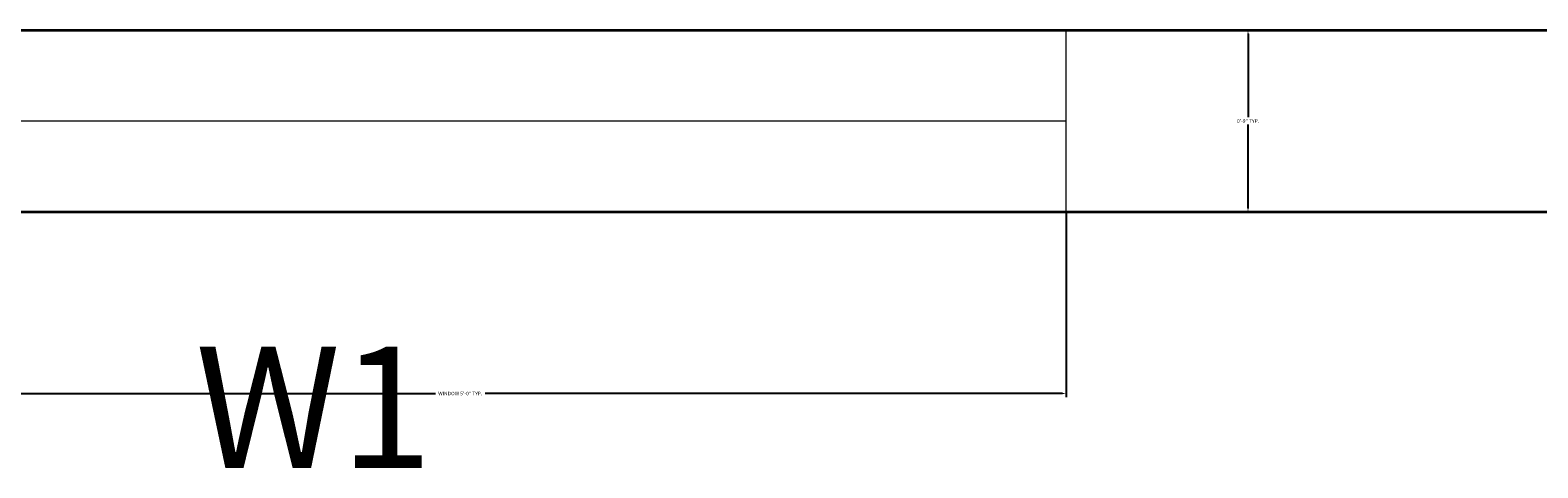
# Model space of a CAD drawing. Units: inches. Extents: x -36302355 to 648, y -221479757 to 75.
# Tile 16 of 37: x 516 to 591, y -593 to -571. Entities that reach past the tile are written whole.
import ezdxf

# ---------------------------------------------------------------- set-up
doc = ezdxf.new("R2010")
doc.units = ezdxf.units.IN
doc.header["$MEASUREMENT"] = 0
for name, color, linetype, lineweight in [('A-ANNO-DIMS', 2, 'Continuous', 18), ('A-ANNO-IDEN', 7, 'Continuous', 18), ('A-GLAZ', 142, 'Continuous', 18), ('A-WALL', 7, 'Continuous', 35)]:
    doc.layers.add(name, color=color, linetype=linetype, lineweight=lineweight)
doc.styles.get("Standard").update_dxf_attribs({"font": 'arial.ttf'})
doc.dimstyles.get("Standard").update_dxf_attribs({"dimtxt": 0.18, "dimasz": 0.18, "dimexe": 0.18, "dimexo": 0.0625, "dimgap": 0.09, "dimtad": 0, "dimtih": 1, "dimtoh": 1, "dimdec": 0, "dimzin": 0, "dimdsep": 46, "dimlunit": 3, "dimtxsty": 'Standard', "dimcen": 0.09, "dimadec": 0, "dimazin": 0, "dimtfac": 1, "dimtdec": 0, "dimtofl": 0, "dimtmove": 0, "dimatfit": 3, "dimfxl": 1, "dimtolj": 1, "dimtzin": 0, "dimarcsym": 0})

# ---------------------------------------------------------------- blocks, each defined once
blk = doc.blocks.new('WIN-60')
for p, q in [((60, 9), (0, 9)), ((0, 9), (0, 0)), ((60, 0), (60, 9)), ((0, 4.5), (60, 4.5)), ((0, 0), (60, 0))]:
    blk.add_line(p, q)
blk = doc.blocks.new('*D23')
at = {"layer": 'A-ANNO-DIMS', "color": 0, "lineweight": -2, "transparency": 16777216}
for p, q in [((507.513, -580.082), (507.513, -589.199)), ((567.513, -580.082), (567.513, -589.199)), ((507.693, -589.019), (536.284, -589.019)), ((567.333, -589.019), (538.742, -589.019))]:
    blk.add_line(p, q, dxfattribs=at)
at = {"layer": 'A-ANNO-DIMS', "color": 0, "transparency": 16777216}
for points in [[(507.693, -588.989), (507.693, -589.049), (507.513, -589.019)], [(567.333, -588.989), (567.333, -589.049), (567.513, -589.019)]]:
    blk.add_solid(points, dxfattribs=at)
at = {"layer": 'Defpoints', "color": 0, "transparency": 16777216}
for p in [(507.513, -580.019), (567.513, -580.019), (567.513, -589.019)]:
    blk.add_point(p, dxfattribs=at)
at = {"layer": 'A-ANNO-DIMS', "color": 0, "transparency": 16777216, "insert": (537.513, -589.019), "char_height": 0.18, "attachment_point": 5}
blk.add_mtext('\\A1;WINDOW 5\'-0" TYP.', dxfattribs=at)
blk = doc.blocks.new('*D24')
at = {"layer": 'A-ANNO-DIMS', "color": 0, "lineweight": -2, "transparency": 16777216}
for p, q in [((567.575, -571.019), (576.693, -571.019)), ((576.513, -571.199), (576.513, -575.337)), ((576.513, -579.839), (576.513, -575.701)), ((567.575, -580.019), (576.693, -580.019))]:
    blk.add_line(p, q, dxfattribs=at)
at = {"layer": 'A-ANNO-DIMS', "color": 0, "transparency": 16777216}
for points in [[(576.483, -571.199), (576.543, -571.199), (576.513, -571.019)], [(576.483, -579.839), (576.543, -579.839), (576.513, -580.019)]]:
    blk.add_solid(points, dxfattribs=at)
at = {"layer": 'Defpoints', "color": 0, "transparency": 16777216}
for p in [(567.513, -571.019), (576.513, -571.019), (567.513, -580.019)]:
    blk.add_point(p, dxfattribs=at)
at = {"layer": 'A-ANNO-DIMS', "color": 0, "transparency": 16777216, "insert": (576.513, -575.519), "char_height": 0.18, "attachment_point": 5}
blk.add_mtext('\\A1;0\'-9" TYP.', dxfattribs=at)

msp = doc.modelspace()

# ---------------------------------------------------------------- linework, layer by layer
at = {"layer": 'A-WALL'}
for p, q in [((335.197, -571.019), (605.197, -571.019)), ((335.197, -580.019), (605.197, -580.019))]:
    msp.add_line(p, q, dxfattribs=at)

# ---------------------------------------------------------------- block references
at = {"layer": 'A-GLAZ'}
msp.add_blockref('WIN-60', (507.513, -580.019), dxfattribs=at)

# ---------------------------------------------------------------- texts
at = {"layer": 'A-ANNO-IDEN', "insert": (524.397, -586.7), "char_height": 6, "attachment_point": 1}
msp.add_mtext_dynamic_manual_height_columns('W1', width=0.80208, gutter_width=1, heights=[0], dxfattribs=at)

# ---------------------------------------------------------------- dimensions: what is measured, and where the dimension line sits
at = {"layer": 'A-ANNO-DIMS'}
dim = msp.add_linear_dim(base=(576.513, -571.019), p1=(567.513, -580.019), p2=(567.513, -571.019), angle=90, text='<> TYP.', dimstyle='Standard', override={"dimdec": 1, "dimlfac": 1, "dimrnd": 0, "dimzin": 1, "dimdsep": 46, "dimlunit": 4, "dimfrac": 2}, dxfattribs=at)
dim.commit()
dim.dimension.update_dxf_attribs({"geometry": '*D24', "text_midpoint": (576.513, -575.519)})
dim = msp.add_linear_dim(base=(567.513, -589.019), p1=(507.513, -580.019), p2=(567.513, -580.019), text='WINDOW <> TYP.', dimstyle='Standard', override={"dimdec": 1, "dimlfac": 1, "dimrnd": 0, "dimzin": 1, "dimdsep": 46, "dimlunit": 4, "dimfrac": 2}, dxfattribs=at)
dim.commit()
dim.dimension.update_dxf_attribs({"geometry": '*D23', "text_midpoint": (537.513, -589.019)})

doc.saveas('drawing.dxf')
